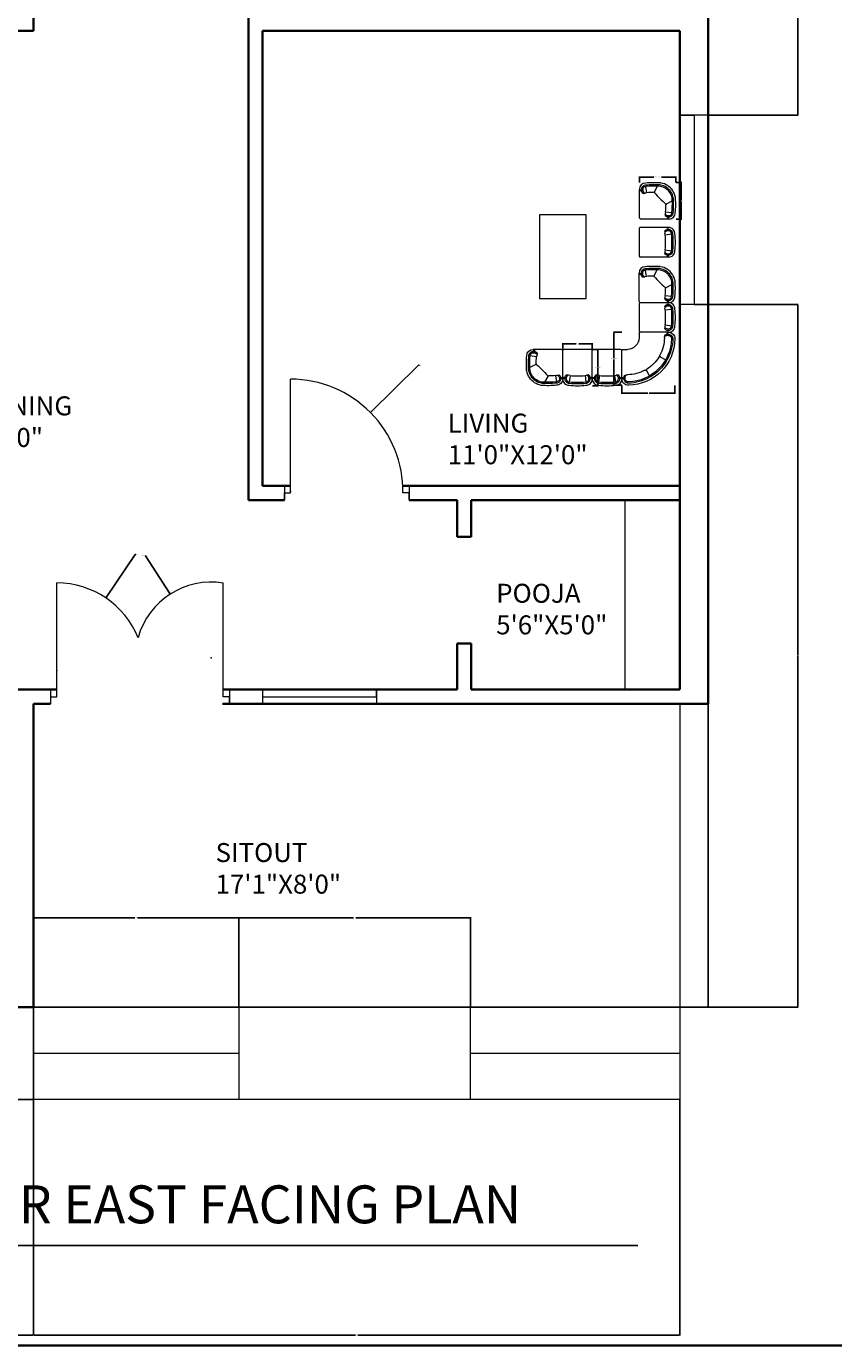
# Model space of a CAD drawing. Units: inches. Extents: x 1832 to 2989, y 1644 to 2902.
# Tile 2 of 8: x 2087 to 2343, y 1644 to 2061. Entities that reach past the tile are written whole.
import ezdxf

# ---------------------------------------------------------------- set-up
doc = ezdxf.new("R2010")
doc.units = ezdxf.units.IN
for name, color, linetype, lineweight in [('A-ANNO-DIMS', 2, 'Continuous', 18), ('A-ANNO-TEXT', 7, 'Continuous', 25), ('A-ANNO-TTLB', 7, 'Continuous', 35), ('A-AREA-IDEN', 7, 'Continuous', 18), ('A-DOOR', 3, 'Continuous', 18), ('A-FLOR', 7, 'Continuous', 25), ('A-FLOR-CASE', 8, 'Continuous', 18), ('A-FLOR-STRS', 7, 'Continuous', 18), ('A-FURN', 8, 'Continuous', 18), ('A-GLAZ', 4, 'Continuous', 18), ('A-WALL', 7, 'Continuous', 35)]:
    doc.layers.add(name, color=color, linetype=linetype, lineweight=lineweight)
doc.styles.get("Standard").update_dxf_attribs({"font": 'arial.ttf'})
doc.dimstyles.get("Standard").update_dxf_attribs({"dimtxt": 0.18, "dimasz": 0.18, "dimexe": 0.18, "dimexo": 0.0625, "dimgap": 0.09, "dimtad": 0, "dimtih": 1, "dimtoh": 1, "dimdec": 4, "dimzin": 0, "dimdsep": 46, "dimtxsty": 'Standard', "dimcen": 0.09, "dimadec": 0, "dimazin": 0, "dimtfac": 1, "dimtdec": 4, "dimtofl": 0, "dimtmove": 0, "dimatfit": 3, "dimfxl": 1, "dimtolj": 1, "dimtzin": 0, "dimarcsym": 0})

# ---------------------------------------------------------------- blocks, each defined once
blk = doc.blocks.new('A$C707258B2')
at = {"color": 0}
for p, q in [((0.404, 0.342), (1.074, 0.342)), ((0.404, 0.292), (0.454, 0.292)), ((0.404, 0.262), (0.454, 0.262)), ((1.104, 0.312), (1.104, 0.212)), ((0.6, -0.238), (0.47, -0.313)), ((1.479, -0.063), (1.379, -0.063)), ((1.509, -0.763), (1.509, -0.093)), ((0.929, -0.567), (0.854, -0.697)), ((1.429, -0.763), (1.429, -0.713)), ((1.459, -0.763), (1.459, -0.712))]:
    blk.add_line(p, q, dxfattribs=at)
for centre, radius, start, end in [((0.404, 0.192), 0.15, 90, 181.1754), ((0.378, 0.317), 0.0362, 316.3972, 43.6028), ((0.368, 0.317), 0.0662, 337.8298, 22.1702), ((1.074, 0.312), 0.03, 360, 90), ((1.379, 0.212), 1.125, 181.1754, 268.8246), ((0.404, 0.192), 0.1, 90, 181.1754), ((1.379, 0.212), 1.075, 181.1754, 208.6357), ((0.404, 0.192), 0.07, 90, 181.1754), ((1.379, 0.212), 1.045, 181.1754, 268.8246), ((0.455, 0.256), 0.0357, 345.4262, 90.5555), ((0.454, 0.212), 0.05, 360, 90), ((1.379, 0.212), 0.875, 180, 208.4082), ((1.379, 0.212), 0.275, 180, 270), ((0.457, -0.291), 0.025, 208.6357, 300), ((0.587, -0.216), 0.025, 300, 28.4082), ((0.612, -0.259), 0.025, 31.5918, 120), ((1.379, 0.212), 0.875, 211.5918, 238.4082), ((1.479, -0.093), 0.03, 360, 90), ((0.482, -0.334), 0.025, 120, 211.3643), ((1.379, 0.212), 1.075, 211.3643, 238.6357), ((0.907, -0.555), 0.025, 330, 58.4082), ((0.951, -0.58), 0.025, 61.5918, 150), ((1.379, 0.212), 0.875, 241.5918, 270), ((0.832, -0.685), 0.025, 238.6357, 330), ((0.876, -0.71), 0.025, 150, 241.3643), ((1.379, 0.212), 1.075, 241.3643, 268.8246), ((1.359, -0.763), 0.15, 268.8246, 360), ((1.359, -0.763), 0.1, 268.8246, 360), ((1.359, -0.763), 0.07, 268.8246, 360), ((1.379, -0.713), 0.05, 360, 90), ((1.425, -0.709), 0.0336, 354.6301, 109.3883), ((1.484, -0.799), 0.0662, 67.8298, 112.1702), ((1.484, -0.789), 0.0362, 46.3972, 133.6028)]:
    blk.add_arc(centre, radius, start, end, dxfattribs=at)
blk = doc.blocks.new('part 01')
at = {"color": 0}
for p, q in [((-670, 700), (0, 700)), ((30, 30), (30, 670)), ((-591, 527), (-740, 550)), ((-591, 527), (-579, 561)), ((-591, 173), (-740, 150)), ((-670, 0), (0, 0)), ((-591, 173), (-579, 139))]:
    blk.add_line(p, q, dxfattribs=at)
for centre, radius, start, end in [((-670, 550), 150, 90, 181.1754), ((-670, 550), 100, 90, 181.1754), ((-660, 518), 133, 56.0897, 95.6132), ((-696, 675), 36.2, 316.3972, 43.6028), ((-706, 675), 66.2, 337.8298, 22.1702), ((-600, 607), 25, 332.9608, 56.0897), ((0, 670), 30, 0, 90), ((1178, 350), 2008, 174.2835, 185.7165), ((1178, 350), 1958, 174.2835, 185.7165), ((1178, 350), 1928, 174.2835, 185.7165), ((-670, 550), 70, 90, 181.1754), ((-660, 518), 103, 42.0066, 95.6132), ((1178, 350), 1778, 174.2835, 185.7165), ((-625, 620), 53.2, 321.0017, 332.9608), ((-602, 570), 25, 340, 42.0066), ((-670, 150), 150, 178.8246, 270), ((-670, 150), 100, 178.8246, 270), ((-670, 150), 70, 178.8246, 270), ((-660, 182), 133, 264.3868, 303.9103), ((-660, 182), 103, 264.3868, 317.9934), ((-696, 25), 36.2, 316.3972, 43.6028), ((-706, 25), 66.2, 337.8298, 22.1702), ((-600, 93), 25, 303.9103, 27.0392), ((-602, 130), 25, 317.9934, 20), ((-625, 80), 53.2, 27.0392, 38.9983), ((0, 30), 30, 270, 0)]:
    blk.add_arc(centre, radius, start, end, dxfattribs=at)
blk = doc.blocks.new('part02')
at = {"color": 0}
for p, q in [((0, -670), (0, 0)), ((30, 30), (700, 30)), ((621, -143), (609, -109)), ((621, -143), (770, -120)), ((173, -591), (139, -579)), ((173, -591), (150, -740)), ((356, -610), (429, -748)), ((640, -326), (778, -399))]:
    blk.add_line(p, q, dxfattribs=at)
for centre, radius, start, end in [((30, 0), 30, 90, 180), ((726, 5), 56.2, 153.6122, 206.6666), ((726, 5), 36.2, 136.3972, 223.6028), ((700, -120), 150, 0, 90), ((630, -63), 25, 123.9103, 207.0392), ((655, -50), 53.2, 207.0392, 218.9983), ((632, -100), 25, 137.9934, 200), ((690, -152), 103, 84.3868, 137.9934), ((689, -151), 132, 85.4378, 123.9887), ((-1148, -320), 1778, 0.3836, 5.7165), ((650, -308), 20, 180.3836, 242), ((700, -121), 101, 357.5006, 89.858), ((700, -120), 70, 0, 90), ((-1228, -320), 2008, 357.7349, 5.7032), ((-1148, -320), 1958, 355.8657, 5.7165), ((-1148, -320), 2008, 355.818, 5.7165), ((182, -660), 133, 146.0897, 185.6132), ((93, -600), 25, 62.9608, 146.0897), ((182, -660), 103, 132.0066, 185.6132), ((80, -625), 53.2, 51.0017, 62.9608), ((130, -602), 25, 70, 132.0066), ((350, 1178), 1778, 264.2835, 269.6164), ((338, -620), 20, 28, 89.6164), ((374, -602), 20, 139.3039, 208), ((2220, -2190), 2454, 130.6961, 139.3039), ((439, -409), 419, 268.2181, 1.7819), ((439, -409), 369, 268.2181, 1.7819), ((439, -409), 339, 268.2181, 1.7819), ((632, -344), 20, 62, 130.6961), ((25, -696), 56.2, 63.3334, 116.3878), ((25, -696), 36.2, 46.3972, 133.6028), ((150, -670), 150, 180, 271.1754), ((150, -670), 100, 180, 271.1754), ((150, -670), 70, 180, 270), ((350, 1258), 2008, 264.2968, 272.2651), ((350, 1178), 2008, 264.2835, 274.182), ((350, 1178), 1958, 264.2835, 274.1343)]:
    blk.add_arc(centre, radius, start, end, dxfattribs=at)
blk = doc.blocks.new('WIN-PLAN-60IN')
for p, q in [((0, 9), (0, 0)), ((60, 4.5), (60, 9)), ((60, 9), (60, 0)), ((0, 0), (0, 4.5)), ((0, 4.5), (60, 4.5))]:
    blk.add_line(p, q)
blk = doc.blocks.new('DOOR-PLAN-ENTRY-PAIR')
for p, q in [((2, 2.25), (2, 38.25)), ((54.64, 2.25), (54.64, 38.25)), ((0, 4.5), (0, 0)), ((56.64, 4.5), (56.64, 0)), ((56.64, 4.5), (56.64, 2.25)), ((0, 2.25), (2, 2.25)), ((56.64, 2.25), (54.64, 2.25)), ((56.64, 0), (56.64, 2.25))]:
    blk.add_line(p, q)
for centre, radius, start, end in [((2, 10.56), 27.69, 21.9895, 90), ((50.82, 14.55), 24, 80.8436, 164.5954)]:
    blk.add_arc(centre, radius, start, end)
blk = doc.blocks.new('DOOR-PLAN-LIVING')
for p, q in [((2, 26.25), (2, 38.25)), ((2, 2.25), (2, 26.25)), ((0, 4.5), (0, 0)), ((39.53, 4.5), (39.53, 0)), ((0, 0), (0, 2.25)), ((0, 2.25), (2, 2.25)), ((39.53, 2.25), (37.53, 2.25)), ((39.53, 0), (39.53, 2.25))]:
    blk.add_line(p, q)
blk.add_arc((2, 2.72), 35.53, 359.2416, 90)
blk = doc.blocks.new('WIN-PLAN-PARTITION-36IN')
for p, q in [((0, 4.5), (0, 0)), ((36, 2.25), (36, 4.5)), ((36, 4.5), (36, 0)), ((0, 2.25), (36, 2.25))]:
    blk.add_line(p, q)
blk = doc.blocks.new('*D31')
at = {"layer": 'A-ANNO-DIMS', "color": 0, "lineweight": -2, "transparency": 16777216}
for p, q in [((2266.26, 1958.86), (2268.11, 1958.86)), ((2267.93, 1958.68), (2267.93, 1953.27)), ((2267.93, 1947.5), (2267.93, 1952.91)), ((2266.26, 1947.32), (2268.11, 1947.32))]:
    blk.add_line(p, q, dxfattribs=at)
at = {"layer": 'A-ANNO-DIMS', "color": 0, "transparency": 16777216}
for points in [[(2267.9, 1958.68), (2267.96, 1958.68), (2267.93, 1958.86)], [(2267.9, 1947.5), (2267.96, 1947.5), (2267.93, 1947.32)]]:
    blk.add_solid(points, dxfattribs=at)
at = {"layer": 'Defpoints', "color": 0, "transparency": 16777216}
for p in [(2266.2, 1958.86), (2267.93, 1958.86), (2266.2, 1947.32)]:
    blk.add_point(p, dxfattribs=at)
at = {"layer": 'A-ANNO-DIMS', "color": 0, "transparency": 16777216, "insert": (2267.93, 1953.09), "char_height": 0.18, "attachment_point": 5}
blk.add_mtext('\\A1;SOFA SEAT 12 TYP.', dxfattribs=at)
blk = doc.blocks.new('*D32')
at = {"layer": 'A-ANNO-DIMS', "color": 0, "lineweight": -2, "transparency": 16777216}
for p, q in [((2256.84, 1958.92), (2256.84, 1960.77)), ((2257.02, 1960.59), (2261.06, 1960.59)), ((2266.02, 1960.59), (2261.98, 1960.59)), ((2266.2, 1958.92), (2266.2, 1960.77))]:
    blk.add_line(p, q, dxfattribs=at)
at = {"layer": 'A-ANNO-DIMS', "color": 0, "transparency": 16777216}
for points in [[(2257.02, 1960.62), (2257.02, 1960.56), (2256.84, 1960.59)], [(2266.02, 1960.62), (2266.02, 1960.56), (2266.2, 1960.59)]]:
    blk.add_solid(points, dxfattribs=at)
at = {"layer": 'Defpoints', "color": 0, "transparency": 16777216}
for p in [(2256.84, 1960.59), (2256.84, 1958.86), (2266.2, 1958.86)]:
    blk.add_point(p, dxfattribs=at)
at = {"layer": 'A-ANNO-DIMS', "color": 0, "transparency": 16777216, "insert": (2261.52, 1960.59), "char_height": 0.18, "attachment_point": 5}
blk.add_mtext('\\A1;9 TYP.', dxfattribs=at)
blk = doc.blocks.new('*D33')
at = {"layer": 'A-ANNO-DIMS', "color": 0, "lineweight": -2, "transparency": 16777216}
for p, q in [((2281.08, 2011.71), (2281.08, 2013.56)), ((2281.26, 2013.38), (2285.65, 2013.38)), ((2292.44, 2013.38), (2288.06, 2013.38)), ((2292.62, 2011.71), (2292.62, 2013.56))]:
    blk.add_line(p, q, dxfattribs=at)
at = {"layer": 'A-ANNO-DIMS', "color": 0, "transparency": 16777216}
for points in [[(2281.26, 2013.41), (2281.26, 2013.35), (2281.08, 2013.38)], [(2292.44, 2013.41), (2292.44, 2013.35), (2292.62, 2013.38)]]:
    blk.add_solid(points, dxfattribs=at)
at = {"layer": 'Defpoints', "color": 0, "transparency": 16777216}
for p in [(2281.08, 2013.38), (2281.08, 2011.65), (2292.62, 2011.65)]:
    blk.add_point(p, dxfattribs=at)
at = {"layer": 'A-ANNO-DIMS', "color": 0, "transparency": 16777216, "insert": (2286.85, 2013.38), "char_height": 0.18, "attachment_point": 5}
blk.add_mtext('\\A1;SOFA END 12 TYP.', dxfattribs=at)
blk = doc.blocks.new('*D34')
at = {"layer": 'A-ANNO-DIMS', "color": 0, "lineweight": -2, "transparency": 16777216}
for p, q in [((2292.68, 2011.65), (2294.53, 2011.65)), ((2294.35, 2011.47), (2294.35, 2006.06)), ((2294.35, 2000.29), (2294.35, 2005.7)), ((2292.68, 2000.11), (2294.53, 2000.11))]:
    blk.add_line(p, q, dxfattribs=at)
at = {"layer": 'A-ANNO-DIMS', "color": 0, "transparency": 16777216}
for points in [[(2294.32, 2011.47), (2294.38, 2011.47), (2294.35, 2011.65)], [(2294.32, 2000.29), (2294.38, 2000.29), (2294.35, 2000.11)]]:
    blk.add_solid(points, dxfattribs=at)
at = {"layer": 'Defpoints', "color": 0, "transparency": 16777216}
for p in [(2292.62, 2011.65), (2294.35, 2011.65), (2292.62, 2000.11)]:
    blk.add_point(p, dxfattribs=at)
at = {"layer": 'A-ANNO-DIMS', "color": 0, "transparency": 16777216, "insert": (2294.35, 2005.88), "char_height": 0.18, "attachment_point": 5}
blk.add_mtext('\\A1;12 TYP.', dxfattribs=at)
blk = doc.blocks.new('*D35')
at = {"layer": 'A-ANNO-DIMS', "color": 0, "lineweight": -2, "transparency": 16777216}
for p, q in [((2275.49, 1964.28), (2272.86, 1964.28)), ((2273.04, 1964.1), (2273.04, 1956.06)), ((2273.04, 1947.67), (2273.04, 1955.7)), ((2275.49, 1947.49), (2272.86, 1947.49))]:
    blk.add_line(p, q, dxfattribs=at)
at = {"layer": 'A-ANNO-DIMS', "color": 0, "transparency": 16777216}
for points in [[(2273.01, 1964.1), (2273.07, 1964.1), (2273.04, 1964.28)], [(2273.01, 1947.67), (2273.07, 1947.67), (2273.04, 1947.49)]]:
    blk.add_solid(points, dxfattribs=at)
at = {"layer": 'Defpoints', "color": 0, "transparency": 16777216}
for p in [(2273.04, 1964.28), (2275.56, 1964.28), (2275.56, 1947.49)]:
    blk.add_point(p, dxfattribs=at)
at = {"layer": 'A-ANNO-DIMS', "color": 0, "transparency": 16777216, "insert": (2273.04, 1955.88), "char_height": 0.18, "attachment_point": 5}
blk.add_mtext('\\A1;CORNER SEAT 17', dxfattribs=at)
blk = doc.blocks.new('*D36')
at = {"layer": 'A-ANNO-DIMS', "color": 0, "lineweight": -2, "transparency": 16777216}
for p, q in [((2275.56, 1947.42), (2275.56, 1944.79)), ((2292.35, 1947.42), (2292.35, 1944.79)), ((2275.74, 1944.97), (2283.74, 1944.97)), ((2292.17, 1944.97), (2284.16, 1944.97))]:
    blk.add_line(p, q, dxfattribs=at)
at = {"layer": 'A-ANNO-DIMS', "color": 0, "transparency": 16777216}
for points in [[(2275.74, 1945), (2275.74, 1944.94), (2275.56, 1944.97)], [(2292.17, 1945), (2292.17, 1944.94), (2292.35, 1944.97)]]:
    blk.add_solid(points, dxfattribs=at)
at = {"layer": 'Defpoints', "color": 0, "transparency": 16777216}
for p in [(2275.56, 1947.49), (2292.35, 1947.49), (2275.56, 1944.97)]:
    blk.add_point(p, dxfattribs=at)
at = {"layer": 'A-ANNO-DIMS', "color": 0, "transparency": 16777216, "insert": (2283.95, 1944.97), "char_height": 0.18, "attachment_point": 5}
blk.add_mtext('\\A1;17', dxfattribs=at)
blk = doc.blocks.new('*D72')
at = {"layer": 'A-ANNO-DIMS', "color": 0, "lineweight": -2, "transparency": 16777216}
for p, q in [((1943.83, 2229.17), (1915.41, 2229.17)), ((1915.59, 2228.99), (1915.59, 1975.53)), ((1915.59, 1721.7), (1915.59, 1975.17)), ((2089.33, 1721.52), (1915.41, 1721.52))]:
    blk.add_line(p, q, dxfattribs=at)
at = {"layer": 'A-ANNO-DIMS', "color": 0, "transparency": 16777216}
for points in [[(1915.56, 2228.99), (1915.62, 2228.99), (1915.59, 2229.17)], [(1915.56, 1721.7), (1915.62, 1721.7), (1915.59, 1721.52)]]:
    blk.add_solid(points, dxfattribs=at)
at = {"layer": 'Defpoints', "color": 0, "transparency": 16777216}
for p in [(1915.59, 2229.17), (1943.89, 2229.17), (2089.39, 1721.52)]:
    blk.add_point(p, dxfattribs=at)
at = {"layer": 'A-ANNO-DIMS', "color": 0, "transparency": 16777216, "insert": (1915.59, 1975.35), "char_height": 0.18, "attachment_point": 5}
blk.add_mtext('\\A1;507.6', dxfattribs=at)
blk = doc.blocks.new('*D73')
at = {"layer": 'A-ANNO-DIMS', "color": 0, "lineweight": -2, "transparency": 16777216}
for p, q in [((2302.95, 1973.01), (2331.37, 1973.01)), ((2331.19, 1972.83), (2331.19, 1862.02)), ((2331.19, 1750.85), (2331.19, 1861.66)), ((2302.95, 1750.67), (2331.37, 1750.67))]:
    blk.add_line(p, q, dxfattribs=at)
at = {"layer": 'A-ANNO-DIMS', "color": 0, "transparency": 16777216}
for points in [[(2331.16, 1972.83), (2331.22, 1972.83), (2331.19, 1973.01)], [(2331.16, 1750.85), (2331.22, 1750.85), (2331.19, 1750.67)]]:
    blk.add_solid(points, dxfattribs=at)
at = {"layer": 'Defpoints', "color": 0, "transparency": 16777216}
for p in [(2302.89, 1973.01), (2331.19, 1973.01), (2302.89, 1750.67)]:
    blk.add_point(p, dxfattribs=at)
at = {"layer": 'A-ANNO-DIMS', "color": 0, "transparency": 16777216, "insert": (2331.19, 1861.84), "char_height": 0.18, "attachment_point": 5}
blk.add_mtext('\\A1;222.33', dxfattribs=at)
blk = doc.blocks.new('*D74')
at = {"layer": 'A-ANNO-DIMS', "color": 0, "lineweight": -2, "transparency": 16777216}
for p, q in [((2302.95, 2120.08), (2331.37, 2120.08)), ((2331.19, 2119.9), (2331.19, 2076.73)), ((2331.19, 2033.19), (2331.19, 2076.36)), ((2302.95, 2033.01), (2331.37, 2033.01))]:
    blk.add_line(p, q, dxfattribs=at)
at = {"layer": 'A-ANNO-DIMS', "color": 0, "transparency": 16777216}
for points in [[(2331.16, 2119.9), (2331.22, 2119.9), (2331.19, 2120.08)], [(2331.16, 2033.19), (2331.22, 2033.19), (2331.19, 2033.01)]]:
    blk.add_solid(points, dxfattribs=at)
at = {"layer": 'Defpoints', "color": 0, "transparency": 16777216}
for p in [(2302.89, 2120.08), (2331.19, 2120.08), (2302.89, 2033.01)]:
    blk.add_point(p, dxfattribs=at)
at = {"layer": 'A-ANNO-DIMS', "color": 0, "transparency": 16777216, "insert": (2331.19, 2076.55), "char_height": 0.18, "attachment_point": 5}
blk.add_mtext('\\A1;87.08', dxfattribs=at)
blk = doc.blocks.new('*D75')
at = {"layer": 'A-ANNO-DIMS', "color": 0, "lineweight": -2, "transparency": 16777216}
for p, q in [((1943.89, 1750.61), (1943.89, 1646.75)), ((2089.39, 1750.61), (2089.39, 1646.75)), ((1944.07, 1646.93), (2016.25, 1646.93)), ((2089.21, 1646.93), (2017.03, 1646.93))]:
    blk.add_line(p, q, dxfattribs=at)
at = {"layer": 'A-ANNO-DIMS', "color": 0, "transparency": 16777216}
for points in [[(1944.07, 1646.96), (1944.07, 1646.9), (1943.89, 1646.93)], [(2089.21, 1646.96), (2089.21, 1646.9), (2089.39, 1646.93)]]:
    blk.add_solid(points, dxfattribs=at)
at = {"layer": 'Defpoints', "color": 0, "transparency": 16777216}
for p in [(1943.89, 1750.67), (2089.39, 1750.67), (2089.39, 1646.93)]:
    blk.add_point(p, dxfattribs=at)
at = {"layer": 'A-ANNO-DIMS', "color": 0, "transparency": 16777216, "insert": (2016.64, 1646.93), "char_height": 0.18, "attachment_point": 5}
blk.add_mtext('\\A1;145.5', dxfattribs=at)
blk = doc.blocks.new('*D76')
at = {"layer": 'A-ANNO-DIMS', "color": 0, "lineweight": -2, "transparency": 16777216}
for p, q in [((2089.39, 1721.46), (2089.39, 1646.75)), ((2293.89, 1721.46), (2293.89, 1646.75)), ((2089.57, 1646.93), (2191.24, 1646.93)), ((2293.71, 1646.93), (2192.04, 1646.93))]:
    blk.add_line(p, q, dxfattribs=at)
at = {"layer": 'A-ANNO-DIMS', "color": 0, "transparency": 16777216}
for points in [[(2089.57, 1646.96), (2089.57, 1646.9), (2089.39, 1646.93)], [(2293.71, 1646.96), (2293.71, 1646.9), (2293.89, 1646.93)]]:
    blk.add_solid(points, dxfattribs=at)
at = {"layer": 'Defpoints', "color": 0, "transparency": 16777216}
for p in [(2089.39, 1721.52), (2293.89, 1721.52), (2293.89, 1646.93)]:
    blk.add_point(p, dxfattribs=at)
at = {"layer": 'A-ANNO-DIMS', "color": 0, "transparency": 16777216, "insert": (2191.64, 1646.93), "char_height": 0.18, "attachment_point": 5}
blk.add_mtext('\\A1;204.5', dxfattribs=at)
blk = doc.blocks.new('*D77')
at = {"layer": 'A-ANNO-DIMS', "color": 0, "lineweight": -2, "transparency": 16777216}
for p, q in [((2089.39, 1750.74), (2089.39, 1779.15)), ((2089.57, 1778.97), (2121.49, 1778.97)), ((2154.2, 1778.97), (2122.28, 1778.97)), ((2154.38, 1750.74), (2154.38, 1779.15))]:
    blk.add_line(p, q, dxfattribs=at)
at = {"layer": 'A-ANNO-DIMS', "color": 0, "transparency": 16777216}
for points in [[(2089.57, 1779), (2089.57, 1778.94), (2089.39, 1778.97)], [(2154.2, 1779), (2154.2, 1778.94), (2154.38, 1778.97)]]:
    blk.add_solid(points, dxfattribs=at)
at = {"layer": 'Defpoints', "color": 0, "transparency": 16777216}
for p in [(2154.38, 1778.97), (2089.39, 1750.67), (2154.38, 1750.67)]:
    blk.add_point(p, dxfattribs=at)
at = {"layer": 'A-ANNO-DIMS', "color": 0, "transparency": 16777216, "insert": (2121.88, 1778.97), "char_height": 0.18, "attachment_point": 5}
blk.add_mtext('\\A1;64.99', dxfattribs=at)
blk = doc.blocks.new('*D78')
at = {"layer": 'A-ANNO-DIMS', "color": 0, "lineweight": -2, "transparency": 16777216}
for p, q in [((2154.38, 1750.74), (2154.38, 1779.15)), ((2154.56, 1778.97), (2190.62, 1778.97)), ((2227.46, 1778.97), (2191.4, 1778.97)), ((2227.64, 1750.74), (2227.64, 1779.15))]:
    blk.add_line(p, q, dxfattribs=at)
at = {"layer": 'A-ANNO-DIMS', "color": 0, "transparency": 16777216}
for points in [[(2154.56, 1779), (2154.56, 1778.94), (2154.38, 1778.97)], [(2227.46, 1779), (2227.46, 1778.94), (2227.64, 1778.97)]]:
    blk.add_solid(points, dxfattribs=at)
at = {"layer": 'Defpoints', "color": 0, "transparency": 16777216}
for p in [(2227.64, 1778.97), (2154.38, 1750.67), (2227.64, 1750.67)]:
    blk.add_point(p, dxfattribs=at)
at = {"layer": 'A-ANNO-DIMS', "color": 0, "transparency": 16777216, "insert": (2191.01, 1778.97), "char_height": 0.18, "attachment_point": 5}
blk.add_mtext('\\A1;73.26', dxfattribs=at)
blk = doc.blocks.new('*D123')
at = {"layer": 'A-ANNO-DIMS', "color": 0, "lineweight": -2, "transparency": 16777216}
for p, q in [((2211.21, 1953.82), (2196.17, 1938.98)), ((2211.39, 1953.82), (2211.21, 1953.82)), ((2170.66, 1913.89), (2170.84, 1913.89)), ((2170.75, 1913.8), (2170.75, 1913.98))]:
    blk.add_line(p, q, dxfattribs=at)
at = {"layer": 'A-ANNO-DIMS', "color": 0, "transparency": 16777216}
blk.add_solid([(2196.15, 1939), (2196.19, 1938.95), (2196.04, 1938.85)], dxfattribs=at)
at = {"layer": 'Defpoints', "color": 0, "transparency": 16777216}
for p in [(2196.04, 1938.85), (2170.75, 1913.89)]:
    blk.add_point(p, dxfattribs=at)
at = {"layer": 'A-ANNO-DIMS', "color": 0, "transparency": 16777216, "insert": (2211.87, 1953.82), "char_height": 0.18, "attachment_point": 5}
blk.add_mtext('\\A1;R35.53', dxfattribs=at)
blk = doc.blocks.new('*D124')
at = {"layer": 'A-ANNO-DIMS', "color": 0, "lineweight": -2, "transparency": 16777216}
for p, q in [((2121.57, 1893.96), (2112.38, 1880.34)), ((2121.75, 1893.96), (2121.57, 1893.96)), ((2096.71, 1857.23), (2096.89, 1857.23)), ((2096.8, 1857.14), (2096.8, 1857.32))]:
    blk.add_line(p, q, dxfattribs=at)
at = {"layer": 'A-ANNO-DIMS', "color": 0, "transparency": 16777216}
blk.add_solid([(2112.36, 1880.35), (2112.41, 1880.32), (2112.28, 1880.19)], dxfattribs=at)
at = {"layer": 'Defpoints', "color": 0, "transparency": 16777216}
for p in [(2112.28, 1880.19), (2096.8, 1857.23)]:
    blk.add_point(p, dxfattribs=at)
at = {"layer": 'A-ANNO-DIMS', "color": 0, "transparency": 16777216, "insert": (2122.23, 1893.96), "char_height": 0.18, "attachment_point": 5}
blk.add_mtext('\\A1;R27.69', dxfattribs=at)
blk = doc.blocks.new('*D125')
at = {"layer": 'A-ANNO-DIMS', "color": 0, "lineweight": -2, "transparency": 16777216}
for p, q in [((2124.68, 1893.54), (2124.86, 1893.54)), ((2124.86, 1893.54), (2132.54, 1881.57)), ((2145.52, 1861.22), (2145.7, 1861.22)), ((2145.61, 1861.13), (2145.61, 1861.31))]:
    blk.add_line(p, q, dxfattribs=at)
at = {"layer": 'A-ANNO-DIMS', "color": 0, "transparency": 16777216}
blk.add_solid([(2132.57, 1881.59), (2132.52, 1881.56), (2132.64, 1881.42)], dxfattribs=at)
at = {"layer": 'Defpoints', "color": 0, "transparency": 16777216}
for p in [(2132.64, 1881.42), (2145.61, 1861.22)]:
    blk.add_point(p, dxfattribs=at)
at = {"layer": 'A-ANNO-DIMS', "color": 0, "transparency": 16777216, "insert": (2124.12, 1893.54), "char_height": 0.18, "attachment_point": 5}
blk.add_mtext('\\A1;R24.005', dxfattribs=at)

msp = doc.modelspace()

# ---------------------------------------------------------------- linework, layer by layer
at = {"layer": 'A-ANNO-TEXT'}
msp.add_line((1962.8459, 1675.2337), (2280.5653, 1675.2337), dxfattribs=at)
at = {"layer": 'A-ANNO-TTLB'}
msp.add_lwpolyline([(1831.6677, 2901.9044), (2988.9144, 2901.9044), (2988.9144, 1643.5851), (1831.6677, 1643.5851)], close=True, dxfattribs=at)
at = {"layer": 'A-FLOR'}
for p, q in [((2302.8904, 1846.6726), (2302.8904, 1750.6726)), ((2302.8904, 1750.6726), (2089.3904, 1750.6726))]:
    msp.add_line(p, q, dxfattribs=at)
at = {"layer": 'A-FLOR-CASE'}
msp.add_line((2276.5152, 1911.1726), (2276.5152, 1851.1726), dxfattribs=at)
at = {"layer": 'A-FLOR-STRS'}
for p, q in [((2293.8904, 1846.6726), (2293.8904, 1721.5243)), ((2089.3904, 1750.6726), (2089.3904, 1721.5243)), ((2154.3769, 1750.6726), (2154.3769, 1721.5243)), ((2227.639, 1721.5243), (2227.639, 1750.6726)), ((2089.3904, 1736.0984), (2154.3769, 1736.0984)), ((2227.639, 1736.0984), (2293.8904, 1736.0984)), ((2089.3904, 1721.5243), (2293.8904, 1721.5243)), ((2154.3769, 1721.5243), (2227.639, 1721.5243))]:
    msp.add_line(p, q, dxfattribs=at)
at = {"layer": 'A-FURN'}
msp.add_lwpolyline([(2264.279, 2001.4476), (2249.4708, 2001.4476), (2249.4708, 1974.927), (2264.279, 1974.927)], close=True, dxfattribs=at)
at = {"layer": 'A-WALL'}
for p, q in [((2302.8904, 2229.1726), (2302.8904, 1846.6726)), ((2089.3904, 2064.1726), (2089.3904, 2059.6726)), ((2157.3904, 2064.1726), (2157.3904, 2059.6726)), ((2041.3904, 2059.6726), (2089.3904, 2059.6726)), ((2157.3904, 2059.6726), (2157.3904, 1911.1726)), ((2161.8904, 2059.6726), (2293.8904, 2059.6726)), ((2161.8904, 2059.6726), (2161.8904, 1915.6726)), ((2293.8904, 2059.6726), (2293.8904, 1851.1726)), ((2161.8904, 1915.6726), (2170.7521, 1915.6726)), ((2206.2372, 1915.6726), (2293.8904, 1915.6726)), ((2157.3904, 1911.1726), (2168.7521, 1911.1726)), ((2208.2787, 1911.1726), (2223.3904, 1911.1726)), ((2223.3904, 1911.1726), (2223.3904, 1899.525)), ((2227.8904, 1899.525), (2227.8904, 1911.1726)), ((2227.8904, 1911.1726), (2293.8904, 1911.1726)), ((2223.3904, 1899.525), (2227.8904, 1899.525)), ((2223.3904, 1865.7453), (2227.8904, 1865.7453)), ((2223.3904, 1865.7453), (2223.3904, 1851.1726)), ((2227.8904, 1851.1726), (2227.8904, 1865.7453)), ((2075.4242, 1851.1726), (2096.7965, 1851.1726)), ((2149.4347, 1851.1726), (2223.3904, 1851.1726)), ((2223.3904, 1851.1726), (2223.3904, 1851.1726)), ((2293.8904, 1851.1726), (2227.8904, 1851.1726)), ((2227.8904, 1851.1726), (2293.8904, 1851.1726)), ((2089.3904, 1846.6726), (2089.3904, 1759.6726)), ((2089.3904, 1846.6726), (2094.7965, 1846.6726)), ((2161.8904, 1846.6726), (2149.1749, 1846.6726)), ((2161.8904, 1846.6726), (2293.8904, 1846.6726)), ((2293.8904, 1846.6726), (2302.8904, 1846.6726)), ((2089.3904, 1759.6726), (2089.3904, 1750.6726)), ((1952.8904, 1750.6726), (2089.3904, 1750.6726))]:
    msp.add_line(p, q, dxfattribs=at)

# ---------------------------------------------------------------- block references
at = {"layer": 'A-DOOR'}
for name, p in [('DOOR-PLAN-LIVING', (2168.7521, 1911.1726)), ('DOOR-PLAN-ENTRY-PAIR', (2094.7965, 1846.6726))]:
    msp.add_blockref(name, p, dxfattribs=at)
at = {"layer": 'A-FURN', "ltscale": 0.03}
for name, p, xscale, yscale, zscale, rotation in [('part02', (2281.486, 2000.1118), 0.0133711463418911, 0.0133711463418911, 0.0133711463418911, 90), ('part 01', (2281.3739, 1997.4135), 0.0133711463418911, 0.0133711463418911, 0.0133711463418911, 180), ('part02', (2281.3739, 1973.6351), 0.0133711463418911, 0.0133711463418911, 0.0133711463418911, 90), ('part 01', (2281.3739, 1973.6351), 0.0133711463418911, 0.0133711463418911, 0.0133711463418911, 180), ('A$C707258B2', (2295.7338, 1959.7021), -13.37114634189108, 13.37114634189108, 13.37114634189108, 359.9999999999968), ('part02', (2256.8379, 1958.4589), -0.0133711463418911, 0.0133711463418911, 0.0133711463418911, 359.9999999999968), ('part 01', (2266.1977, 1958.4589), 0.0133711463418911, 0.0133711463418911, 0.0133711463418911, 90), ('part 01', (2275.5575, 1958.4589), 0.0133711463418911, 0.0133711463418911, 0.0133711463418911, 90)]:
    msp.add_blockref(name, p, dxfattribs=dict(at, xscale=xscale, yscale=yscale, zscale=zscale, rotation=rotation))
at = {"layer": 'A-GLAZ', "rotation": 270.0000000000006}
msp.add_blockref('WIN-PLAN-60IN', (2293.8904, 2033.0074), dxfattribs=at)
at = {"layer": 'A-GLAZ'}
msp.add_blockref('WIN-PLAN-PARTITION-36IN', (2161.8904, 1846.6726), dxfattribs=at)

# ---------------------------------------------------------------- texts
at = {"layer": 'A-ANNO-TEXT', "insert": (1970.1351, 1694.2857), "char_height": 12, "attachment_point": 1}
msp.add_mtext_dynamic_manual_height_columns('GROUND FLOOR EAST FACING PLAN', width=528.005294, gutter_width=12.5, heights=[0], dxfattribs=at)
at = {"layer": 'A-AREA-IDEN', "char_height": 6, "attachment_point": 1}
for s, width, insert in [('STAIR\\\\DINING\\P17\'1"X13\'0"', 222.625783, (2048.147, 1943.978)), ('LIVING\\P11\'0"X12\'0"', 79.814015, (2220.4439, 1938.5078)), ('POOJA\\P5\'6"X5\'0"', 90.859824, (2235.7806, 1884.6708)), ('SITOUT\\P17\'1"X8\'0"', 153.58108, (2147.0022, 1802.6215))]:
    msp.add_mtext_dynamic_manual_height_columns(s, width=width, gutter_width=12.5, heights=[0], dxfattribs=dict(at, insert=insert))

# ---------------------------------------------------------------- dimensions: what is measured, and where the dimension line sits
at = {"layer": 'A-ANNO-DIMS'}
for base, p1, p2, angle, override, picture, middle in [((1915.5904, 2229.1726), (2089.3904, 1721.5243), (1943.8904, 2229.1726), 90, {"dimdec": 1, "dimlfac": 1, "dimrnd": 0, "dimzin": 0, "dimdsep": 46, "dimlunit": 2}, '*D72', (1915.5904, 1975.3484)), ((2331.1904, 2120.0845), (2302.8904, 2033.0074), (2302.8904, 2120.0845), 90, {"dimdec": 2, "dimlfac": 1, "dimrnd": 0, "dimzin": 0, "dimdsep": 46, "dimlunit": 2}, '*D74', (2331.1904, 2076.546)), ((2331.1904, 1973.0074), (2302.8904, 1750.6726), (2302.8904, 1973.0074), 90, {"dimdec": 2, "dimlfac": 1, "dimrnd": 0, "dimzin": 0, "dimdsep": 46, "dimlunit": 2}, '*D73', (2331.1904, 1861.84)), ((2275.5575, 1944.9683), (2292.3462, 1947.4866), (2275.5575, 1947.4866), 180, {"dimdec": 0, "dimlfac": 1, "dimrnd": 0, "dimzin": 0, "dimdsep": 46, "dimlunit": 2}, '*D36', (2283.9518, 1944.9683)), ((2154.3769, 1778.9726), (2089.3904, 1750.6726), (2154.3769, 1750.6726), 0, {"dimdec": 2, "dimlfac": 1, "dimrnd": 0, "dimzin": 0, "dimdsep": 46, "dimlunit": 2}, '*D77', (2121.8836, 1778.9726))]:
    dim = msp.add_linear_dim(base=base, p1=p1, p2=p2, angle=angle, dimstyle='Standard', override=override, dxfattribs=at)
    dim.commit()
    dim.dimension.update_dxf_attribs({"geometry": picture, "text_midpoint": middle})
for base, p1, p2, angle, text, picture, middle in [((2281.0849, 2013.3801), (2292.6225, 2011.6494), (2281.0849, 2011.6494), 180, 'SOFA END <> TYP.', '*D33', (2286.8537, 2013.3801)), ((2294.3531, 2011.6494), (2292.6225, 2000.1118), (2292.6225, 2011.6494), 90, '<> TYP.', '*D34', (2294.3531, 2005.8806)), ((2273.0392, 1964.2753), (2275.5575, 1947.4866), (2275.5575, 1964.2753), 90, 'CORNER SEAT <>', '*D35', (2273.0392, 1955.881)), ((2256.8379, 1960.5911), (2266.1977, 1958.86), (2256.8379, 1958.86), 180, '<> TYP.', '*D32', (2261.5178, 1960.5911)), ((2267.9288, 1958.86), (2266.1977, 1947.3192), (2266.1977, 1958.86), 90, 'SOFA SEAT <> TYP.', '*D31', (2267.9288, 1953.0896))]:
    dim = msp.add_linear_dim(base=base, p1=p1, p2=p2, angle=angle, text=text, dimstyle='Standard', override={"dimdec": 0, "dimlfac": 1, "dimrnd": 0, "dimzin": 0, "dimdsep": 46, "dimlunit": 2}, dxfattribs=at)
    dim.commit()
    dim.dimension.update_dxf_attribs({"geometry": picture, "text_midpoint": middle})
for center, mpoint, override, picture, middle in [((2170.7521, 1913.8928), (2196.0412, 1938.8492), {"dimdec": 2, "dimlfac": 1, "dimrnd": 0, "dimzin": 0, "dimdsep": 46, "dimlunit": 2}, '*D123', (2211.8745, 1953.823)), ((2096.7965, 1857.2319), (2112.283, 1880.187), {"dimdec": 2, "dimlfac": 1, "dimrnd": 0, "dimzin": 0, "dimdsep": 46, "dimlunit": 2}, '*D124', (2122.235, 1893.9601)), ((2145.6148, 1861.2239), (2132.6401, 1881.4198), {"dimdec": 3, "dimlfac": 1, "dimrnd": 0, "dimzin": 0, "dimdsep": 46, "dimlunit": 2}, '*D125', (2124.1249, 1893.5374))]:
    dim = msp.add_radius_dim(center=center, mpoint=mpoint, dimstyle='Standard', override=override, dxfattribs=at)
    dim.commit()
    dim.dimension.update_dxf_attribs({"geometry": picture, "text_midpoint": middle, "dimtype": 164})
for base, p1, p2, override, picture, middle in [((2227.639, 1778.9726), (2154.3769, 1750.6726), (2227.639, 1750.6726), {"dimdec": 2, "dimlfac": 1, "dimrnd": 0, "dimzin": 0, "dimdsep": 46, "dimlunit": 2}, '*D78', (2191.0079, 1778.9726)), ((2089.3904, 1646.9337), (1943.8904, 1750.6726), (2089.3904, 1750.6726), {"dimdec": 1, "dimlfac": 1, "dimrnd": 0, "dimzin": 0, "dimdsep": 46, "dimlunit": 2}, '*D75', (2016.6404, 1646.9337)), ((2293.8904, 1646.9337), (2089.3904, 1721.5243), (2293.8904, 1721.5243), {"dimdec": 1, "dimlfac": 1, "dimrnd": 0, "dimzin": 0, "dimdsep": 46, "dimlunit": 2}, '*D76', (2191.6404, 1646.9337))]:
    dim = msp.add_linear_dim(base=base, p1=p1, p2=p2, dimstyle='Standard', override=override, dxfattribs=at)
    dim.commit()
    dim.dimension.update_dxf_attribs({"geometry": picture, "text_midpoint": middle})

doc.saveas('drawing.dxf')
